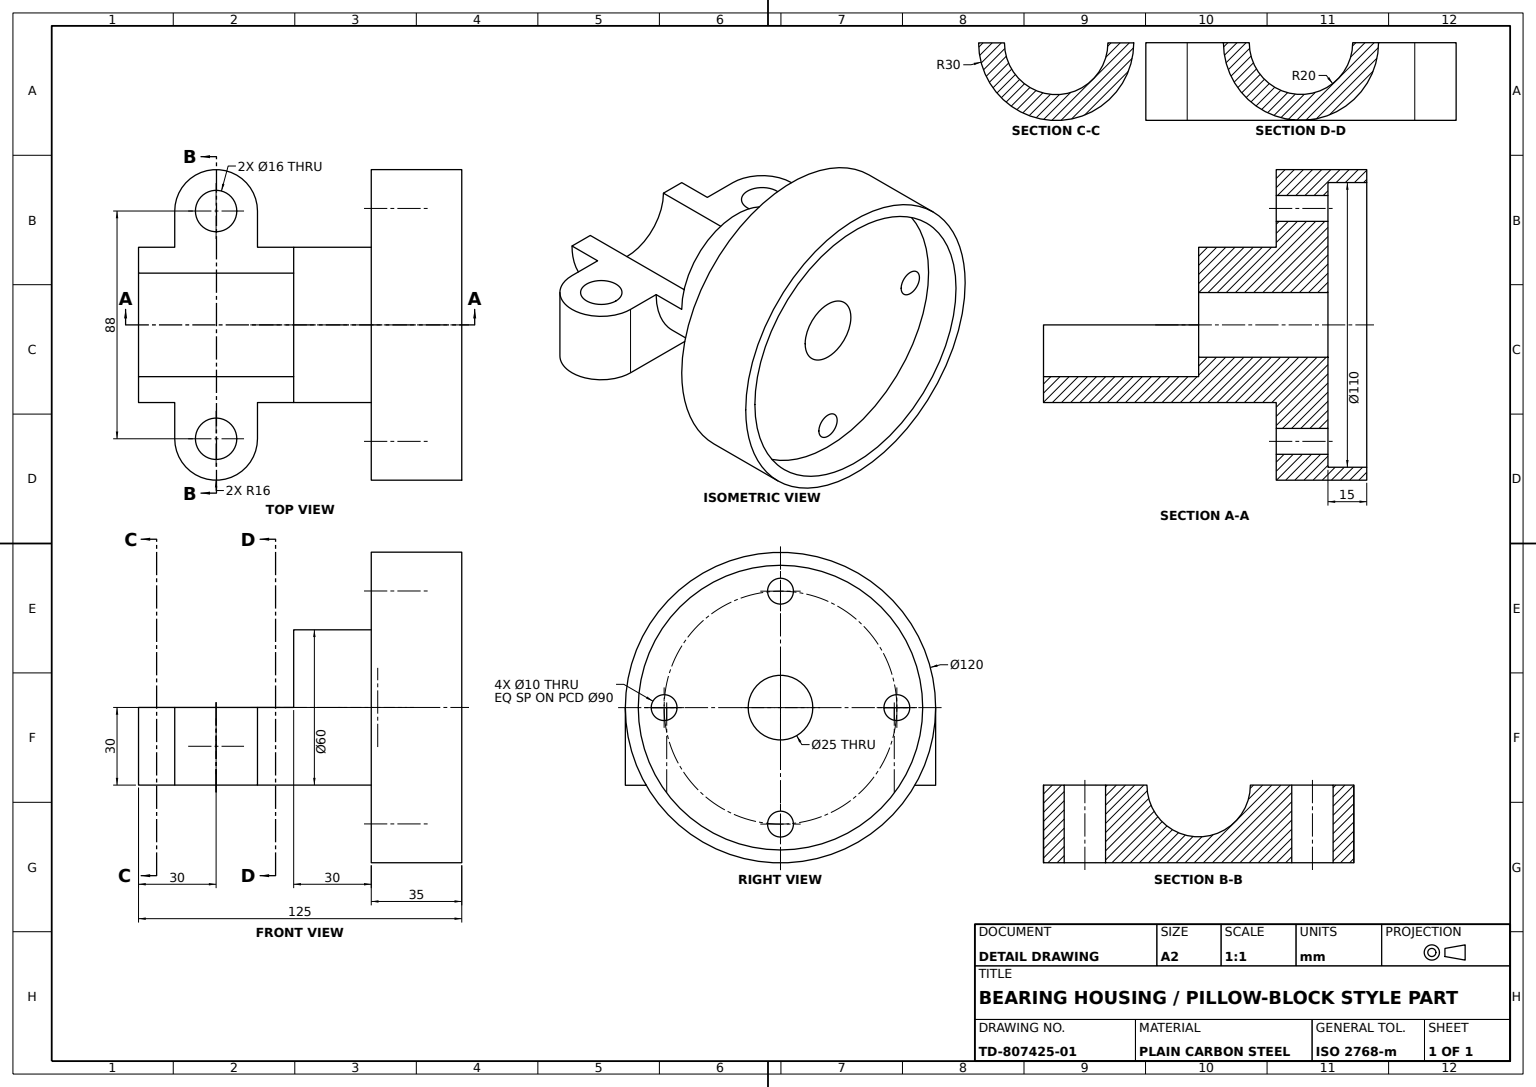
from build123d import *

# Parameters (mm, degrees)
FLANGE_PROFILE_R            = 60
FLANGE_120_DEPTH            = 35
HUB_PROFILE_R               = 30
HUB_DEPTH                   = 30
HALF_BEARING_SADDLE_DEPTH   = 60
FLANGE_RECESS_PROFILE_R     = 55
FLANGE_RECESS_110_DEPTH     = 15
FLANGE_BOLT_HOLES_PROFILE_R = 5
FLANGE_BOLT_HOLES_DEPTH     = 52
SADDLE_BORE_R20_DEPTH       = 60
SHAFT_BORE_PROFILE_R        = 12.5
SHAFT_BORE_25_DEPTH         = 60
MOUNTING_LUG_A_DEPTH        = 30
MOUNTING_LUG_B_DEPTH        = 30
LUG_BRIDGE_PROFILE_W        = 60
LUG_BRIDGE_PROFILE_H        = 32
LUG_BRIDGE_DEPTH            = 30
BRIDGE_BORE_RELIEF_DEPTH    = 35
LUG_HOLES_PROFILE_R         = 8
LUG_HOLES_2X_16_DEPTH       = 35


with BuildPart() as part:
    # Flange Profile → Flange Ø120 (new body)
    with BuildSketch(Plane.XY):
        Circle(FLANGE_PROFILE_R)
    extrude(amount=-FLANGE_120_DEPTH)

    # Hub Profile → Hub (add)
    with BuildSketch(Plane.XY):
        Circle(HUB_PROFILE_R)
    extrude(amount=HUB_DEPTH)

    # Saddle Profile → Half-Bearing Saddle (add)
    with BuildSketch(Plane.XY.offset(30)):
        with BuildLine():
            Line((-30, 0), (30, 0))
            ThreePointArc((30, 0), (0, -30), (-30, 0))
        make_face()
    extrude(amount=HALF_BEARING_SADDLE_DEPTH)

    # Flange Recess Profile → Flange Recess Ø110 (cut)
    with BuildSketch(Plane(origin=(0, 0, -35), x_dir=(-1, 0, 0), z_dir=(0, 0, -1))):
        Circle(FLANGE_RECESS_PROFILE_R)
    extrude(amount=-FLANGE_RECESS_110_DEPTH, mode=Mode.SUBTRACT)

    # Flange Bolt Holes Profile → Flange Bolt Holes (cut)
    with BuildSketch(Plane.XY):
        with Locations((45, 0)):
            Circle(FLANGE_BOLT_HOLES_PROFILE_R)
        with Locations((0, 45)):
            Circle(FLANGE_BOLT_HOLES_PROFILE_R)
        with Locations((-45, 0)):
            Circle(FLANGE_BOLT_HOLES_PROFILE_R)
        with Locations((0, -45)):
            Circle(FLANGE_BOLT_HOLES_PROFILE_R)
    extrude(amount=-FLANGE_BOLT_HOLES_DEPTH, mode=Mode.SUBTRACT)

    # Saddle Bore Profile → Saddle Bore R20 (cut)
    with BuildSketch(Plane.XY.offset(90)):
        with BuildLine():
            Line((-20, 0), (20, 0))
            ThreePointArc((20, 0), (0, -20), (-20, 0))
        make_face()
    extrude(amount=-SADDLE_BORE_R20_DEPTH, mode=Mode.SUBTRACT)

    # Shaft Bore Profile → Shaft Bore Ø25 (cut)
    with BuildSketch(Plane.XY.offset(30)):
        Circle(SHAFT_BORE_PROFILE_R)
    extrude(amount=-SHAFT_BORE_25_DEPTH, mode=Mode.SUBTRACT)



with BuildPart() as body_2:
    # Mounting Lug A Profile → Mounting Lug A (new body)
    with BuildSketch(Plane(origin=(0, 0, 0), x_dir=(1, 0, 0), z_dir=(0, 1, 0))):
        with BuildLine():
            Line((-44, -76), (-30, -76))
            Line((-30, -76), (-30, -44))
            Line((-30, -44), (-44, -44))
            ThreePointArc((-44, -44), (-60, -60), (-44, -76))
        make_face()
    extrude(amount=-MOUNTING_LUG_A_DEPTH)


with BuildPart() as body_3:
    # Mounting Lug B Profile → Mounting Lug B (new body)
    with BuildSketch(Plane(origin=(0, 0, 0), x_dir=(1, 0, 0), z_dir=(0, 1, 0))):
        with BuildLine():
            Line((44, -44), (30, -44))
            Line((30, -44), (30, -76))
            Line((30, -76), (44, -76))
            ThreePointArc((44, -76), (60, -60), (44, -44))
        make_face()
    extrude(amount=-MOUNTING_LUG_B_DEPTH)


with BuildPart() as part_1:
    add(part.part)

    add(body_2.part)  # Lug Bridge merges body 2

    add(body_3.part)  # Lug Bridge merges body 3
    # Lug Bridge Profile → Lug Bridge (add)
    with BuildSketch(Plane.XZ.offset(30)):
        with Locations((0, 60)):
            Rectangle(LUG_BRIDGE_PROFILE_W, LUG_BRIDGE_PROFILE_H)
    extrude(amount=-LUG_BRIDGE_DEPTH)

    # Bridge Relief Profile → Bridge Bore Relief (cut)
    with BuildSketch(Plane.XY.offset(76)):
        with BuildLine():
            Line((-20, 0), (20, 0))
            ThreePointArc((20, 0), (0, -20), (-20, 0))
        make_face()
    extrude(amount=-BRIDGE_BORE_RELIEF_DEPTH, mode=Mode.SUBTRACT)

    # Lug Holes Profile → Lug Holes 2xØ16 (cut)
    with BuildSketch(Plane(origin=(0, 0, 0), x_dir=(1, 0, 0), z_dir=(0, 1, 0))):
        with Locations(Location((-44, -60, 0), (0, 0, 270))):
            Circle(LUG_HOLES_PROFILE_R)
        with Locations(Location((44, -60, 0), (0, 0, 270))):
            Circle(LUG_HOLES_PROFILE_R)
    extrude(amount=-LUG_HOLES_2X_16_DEPTH, mode=Mode.SUBTRACT)


solid = part_1.part
